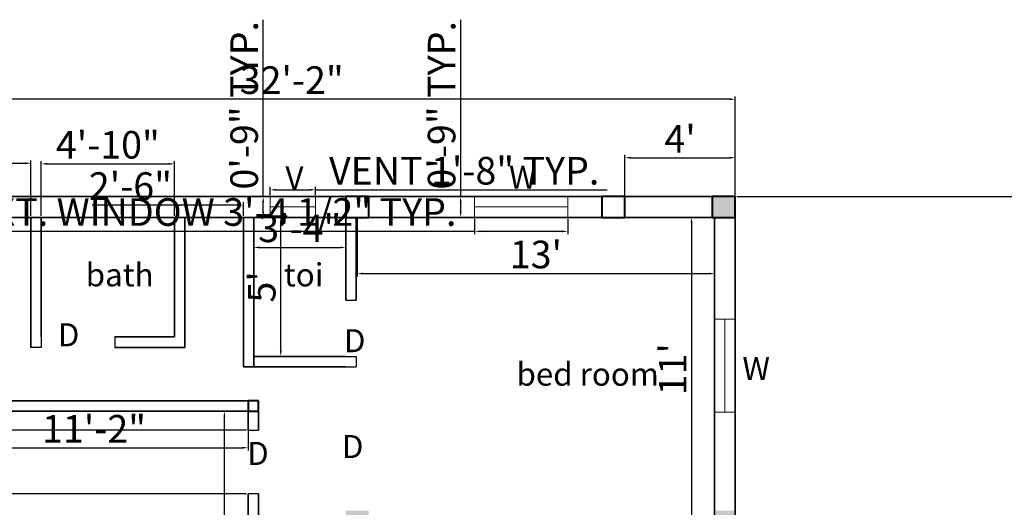
# Model space of a CAD drawing. Units: inches. Extents: x 1989 to 3287, y 1752 to 2384.
# Tile 3 of 5: x 2209 to 2638, y 2172 to 2384. Entities that reach past the tile are written whole.
import ezdxf

# ---------------------------------------------------------------- set-up
doc = ezdxf.new("R2010")
doc.units = ezdxf.units.IN
for name, color, linetype, lineweight in [('A-ANNO-DIMS', 2, 'Continuous', 18), ('A-ANNO-TEXT', 7, 'Continuous', 18), ('A-AREA-IDEN', 7, 'Continuous', 18), ('A-COLS', 1, 'Continuous', 40), ('A-COLS-PATT', 8, 'Continuous', 13), ('A-DOOR', 3, 'Continuous', 25), ('A-GLAZ', 4, 'Continuous', 18), ('A-WALL', 7, 'Continuous', 35)]:
    doc.layers.add(name, color=color, linetype=linetype, lineweight=lineweight)
doc.styles.get("Standard").update_dxf_attribs({"font": 'arial.ttf'})
doc.dimstyles.new('ISO-25', dxfattribs={"dimtxt": 12, "dimasz": 2.5, "dimexe": 1.25, "dimexo": 0.625, "dimtad": 1, "dimdec": 0, "dimlunit": 4, "dimtxsty": 'Standard', "dimcen": 2.5, "dimadec": 0, "dimazin": 0, "dimtfac": 1, "dimtdec": 0, "dimtmove": 0, "dimatfit": 3, "dimfxl": 1, "dimarcsym": 0})

# ---------------------------------------------------------------- blocks, each defined once
blk = doc.blocks.new('*D9')
at = {"layer": 'A-ANNO-DIMS', "color": 0, "lineweight": -2, "transparency": 16777216}
for p, q in [((2308.01, 2213.45), (2297.11, 2213.45)), ((2298.36, 2043.68), (2298.36, 2210.95)), ((2308.01, 2041.18), (2297.11, 2041.18))]:
    blk.add_line(p, q, dxfattribs=at)
at = {"layer": 'A-ANNO-DIMS', "color": 0, "transparency": 16777216}
for points in [[(2297.94, 2210.95), (2298.78, 2210.95), (2298.36, 2213.45)], [(2297.94, 2043.68), (2298.78, 2043.68), (2298.36, 2041.18)]]:
    blk.add_solid(points, dxfattribs=at)
at = {"layer": 'Defpoints', "color": 0, "transparency": 16777216}
for p in [(2298.36, 2213.45), (2308.64, 2213.45), (2308.64, 2041.18)]:
    blk.add_point(p, dxfattribs=at)
at = {"layer": 'A-ANNO-DIMS', "color": 0, "transparency": 16777216, "insert": (2291.71, 2127.31), "char_height": 12, "attachment_point": 5, "rotation": 90}
blk.add_mtext('14\'-4"', dxfattribs=at)
blk = doc.blocks.new('*D10')
at = {"layer": 'A-ANNO-DIMS', "color": 0, "lineweight": -2, "transparency": 16777216}
for p, q in [((2174.64, 2212.82), (2174.64, 2196.3)), ((2308.64, 2212.82), (2308.64, 2196.3)), ((2177.14, 2197.55), (2306.14, 2197.55))]:
    blk.add_line(p, q, dxfattribs=at)
at = {"layer": 'A-ANNO-DIMS', "color": 0, "transparency": 16777216}
for points in [[(2177.14, 2197.97), (2177.14, 2197.13), (2174.64, 2197.55)], [(2306.14, 2197.97), (2306.14, 2197.13), (2308.64, 2197.55)]]:
    blk.add_solid(points, dxfattribs=at)
at = {"layer": 'Defpoints', "color": 0, "transparency": 16777216}
for p in [(2174.64, 2213.45), (2308.64, 2213.45), (2308.64, 2197.55)]:
    blk.add_point(p, dxfattribs=at)
at = {"layer": 'A-ANNO-DIMS', "color": 0, "transparency": 16777216, "insert": (2241.64, 2204.2), "char_height": 12, "attachment_point": 5}
blk.add_mtext('11\'-2"', dxfattribs=at)
blk = doc.blocks.new('*D12')
at = {"layer": 'A-ANNO-DIMS', "color": 0, "lineweight": -2, "transparency": 16777216}
for p, q in [((2134.64, 2307.3), (2134.64, 2350.26)), ((2518.14, 2349.01), (2137.14, 2349.01)), ((2520.64, 2307.3), (2520.64, 2350.26))]:
    blk.add_line(p, q, dxfattribs=at)
at = {"layer": 'A-ANNO-DIMS', "color": 0, "transparency": 16777216}
for points in [[(2137.14, 2349.43), (2137.14, 2348.6), (2134.64, 2349.01)], [(2518.14, 2349.43), (2518.14, 2348.6), (2520.64, 2349.01)]]:
    blk.add_solid(points, dxfattribs=at)
at = {"layer": 'Defpoints', "color": 0, "transparency": 16777216}
for p in [(2134.64, 2349.01), (2134.64, 2306.68), (2520.64, 2306.68)]:
    blk.add_point(p, dxfattribs=at)
at = {"layer": 'A-ANNO-DIMS', "color": 0, "transparency": 16777216, "insert": (2327.64, 2355.77), "char_height": 12, "attachment_point": 5}
blk.add_mtext('32\'-2"', dxfattribs=at)
blk = doc.blocks.new('*D13')
at = {"layer": 'A-ANNO-DIMS', "color": 0, "lineweight": -2, "transparency": 16777216}
for p, q in [((2511.01, 2297.68), (2500.35, 2297.68)), ((2501.6, 2295.18), (2501.6, 2168.18)), ((2511.01, 2165.68), (2500.35, 2165.68))]:
    blk.add_line(p, q, dxfattribs=at)
at = {"layer": 'A-ANNO-DIMS', "color": 0, "transparency": 16777216}
for points in [[(2501.18, 2295.18), (2502.02, 2295.18), (2501.6, 2297.68)], [(2501.18, 2168.18), (2502.02, 2168.18), (2501.6, 2165.68)]]:
    blk.add_solid(points, dxfattribs=at)
at = {"layer": 'Defpoints', "color": 0, "transparency": 16777216}
for p in [(2511.64, 2297.68), (2501.6, 2165.68), (2511.64, 2165.68)]:
    blk.add_point(p, dxfattribs=at)
at = {"layer": 'A-ANNO-DIMS', "color": 0, "transparency": 16777216, "insert": (2494.95, 2231.68), "char_height": 12, "attachment_point": 5, "rotation": 90}
blk.add_mtext("11'", dxfattribs=at)
blk = doc.blocks.new('*D14')
at = {"layer": 'A-ANNO-DIMS', "color": 0, "lineweight": -2, "transparency": 16777216}
for p, q in [((2356.14, 2297.05), (2356.14, 2271.98)), ((2511.64, 2297.05), (2511.64, 2271.98)), ((2358.64, 2273.23), (2509.14, 2273.23))]:
    blk.add_line(p, q, dxfattribs=at)
at = {"layer": 'A-ANNO-DIMS', "color": 0, "transparency": 16777216}
for points in [[(2358.64, 2273.65), (2358.64, 2272.82), (2356.14, 2273.23)], [(2509.14, 2273.65), (2509.14, 2272.82), (2511.64, 2273.23)]]:
    blk.add_solid(points, dxfattribs=at)
at = {"layer": 'Defpoints', "color": 0, "transparency": 16777216}
for p in [(2356.14, 2297.68), (2511.64, 2297.68), (2511.64, 2273.23)]:
    blk.add_point(p, dxfattribs=at)
at = {"layer": 'A-ANNO-DIMS', "color": 0, "transparency": 16777216, "insert": (2433.89, 2279.99), "char_height": 12, "attachment_point": 5}
blk.add_mtext("13'", dxfattribs=at)
blk = doc.blocks.new('*D15')
at = {"layer": 'A-ANNO-DIMS', "color": 0, "lineweight": -2, "transparency": 16777216}
for p, q in [((2311.14, 2297.05), (2311.14, 2283.35)), ((2351.14, 2297.05), (2351.14, 2283.35)), ((2313.64, 2284.6), (2348.64, 2284.6))]:
    blk.add_line(p, q, dxfattribs=at)
at = {"layer": 'A-ANNO-DIMS', "color": 0, "transparency": 16777216}
for points in [[(2313.64, 2285.02), (2313.64, 2284.18), (2311.14, 2284.6)], [(2348.64, 2285.02), (2348.64, 2284.18), (2351.14, 2284.6)]]:
    blk.add_solid(points, dxfattribs=at)
at = {"layer": 'Defpoints', "color": 0, "transparency": 16777216}
for p in [(2311.14, 2297.68), (2351.14, 2297.68), (2351.14, 2284.6)]:
    blk.add_point(p, dxfattribs=at)
at = {"layer": 'A-ANNO-DIMS', "color": 0, "transparency": 16777216, "insert": (2331.14, 2291.36), "char_height": 12, "attachment_point": 5}
blk.add_mtext('3\'-4"', dxfattribs=at)
blk = doc.blocks.new('*D16')
at = {"layer": 'A-ANNO-DIMS', "color": 0, "lineweight": -2, "transparency": 16777216}
for p, q in [((2311.76, 2297.68), (2324.13, 2297.68)), ((2322.88, 2239.73), (2322.88, 2295.18)), ((2311.76, 2237.23), (2324.13, 2237.23))]:
    blk.add_line(p, q, dxfattribs=at)
at = {"layer": 'A-ANNO-DIMS', "color": 0, "transparency": 16777216}
for points in [[(2322.46, 2295.18), (2323.29, 2295.18), (2322.88, 2297.68)], [(2322.46, 2239.73), (2323.29, 2239.73), (2322.88, 2237.23)]]:
    blk.add_solid(points, dxfattribs=at)
at = {"layer": 'Defpoints', "color": 0, "transparency": 16777216}
for p in [(2311.14, 2297.68), (2322.88, 2297.68), (2311.14, 2237.23)]:
    blk.add_point(p, dxfattribs=at)
at = {"layer": 'A-ANNO-DIMS', "color": 0, "transparency": 16777216, "insert": (2316.15, 2267.45), "char_height": 12, "attachment_point": 5, "rotation": 90}
blk.add_mtext("5'", dxfattribs=at)
blk = doc.blocks.new('*D17')
at = {"layer": 'A-ANNO-DIMS', "color": 0, "lineweight": -2, "transparency": 16777216}
for p, q in [((2276.64, 2302.98), (2240.78, 2302.98)), ((2276.64, 2298.3), (2276.64, 2304.23)), ((2304.14, 2302.98), (2279.14, 2302.98)), ((2306.64, 2298.3), (2306.64, 2304.23))]:
    blk.add_line(p, q, dxfattribs=at)
at = {"layer": 'A-ANNO-DIMS', "color": 0, "transparency": 16777216}
for points in [[(2279.14, 2303.4), (2279.14, 2302.56), (2276.64, 2302.98)], [(2304.14, 2303.4), (2304.14, 2302.56), (2306.64, 2302.98)]]:
    blk.add_solid(points, dxfattribs=at)
at = {"layer": 'Defpoints', "color": 0, "transparency": 16777216}
for p in [(2276.64, 2302.98), (2276.64, 2297.68), (2306.64, 2297.68)]:
    blk.add_point(p, dxfattribs=at)
at = {"layer": 'A-ANNO-DIMS', "color": 0, "transparency": 16777216, "insert": (2257.46, 2309.73), "char_height": 12, "attachment_point": 5}
blk.add_mtext('2\'-6"', dxfattribs=at)
blk = doc.blocks.new('*D31')
at = {"layer": 'A-ANNO-DIMS', "color": 0, "lineweight": -2, "transparency": 16777216}
for p, q in [((2166.14, 2298.3), (2166.14, 2322.43)), ((2214.14, 2298.3), (2214.14, 2322.43)), ((2168.64, 2321.18), (2211.64, 2321.18))]:
    blk.add_line(p, q, dxfattribs=at)
at = {"layer": 'A-ANNO-DIMS', "color": 0, "transparency": 16777216}
for points in [[(2168.64, 2321.6), (2168.64, 2320.76), (2166.14, 2321.18)], [(2211.64, 2321.6), (2211.64, 2320.76), (2214.14, 2321.18)]]:
    blk.add_solid(points, dxfattribs=at)
at = {"layer": 'Defpoints', "color": 0, "transparency": 16777216}
for p in [(2214.14, 2321.18), (2166.14, 2297.68), (2214.14, 2297.68)]:
    blk.add_point(p, dxfattribs=at)
at = {"layer": 'A-ANNO-DIMS', "color": 0, "transparency": 16777216, "insert": (2190.14, 2327.8), "char_height": 12, "attachment_point": 5}
blk.add_mtext("4'", dxfattribs=at)
blk = doc.blocks.new('*D33')
at = {"layer": 'A-ANNO-DIMS', "color": 0, "lineweight": -2, "transparency": 16777216}
for p, q in [((2218.64, 2298.3), (2218.64, 2322.17)), ((2276.64, 2298.3), (2276.64, 2322.17)), ((2221.14, 2320.92), (2274.14, 2320.92))]:
    blk.add_line(p, q, dxfattribs=at)
at = {"layer": 'A-ANNO-DIMS', "color": 0, "transparency": 16777216}
for points in [[(2221.14, 2321.33), (2221.14, 2320.5), (2218.64, 2320.92)], [(2274.14, 2321.33), (2274.14, 2320.5), (2276.64, 2320.92)]]:
    blk.add_solid(points, dxfattribs=at)
at = {"layer": 'Defpoints', "color": 0, "transparency": 16777216}
for p in [(2276.64, 2320.92), (2218.64, 2297.68), (2276.64, 2297.68)]:
    blk.add_point(p, dxfattribs=at)
at = {"layer": 'A-ANNO-DIMS', "color": 0, "transparency": 16777216, "insert": (2247.64, 2327.67), "char_height": 12, "attachment_point": 5}
blk.add_mtext('4\'-10"', dxfattribs=at)
blk = doc.blocks.new('*D34')
at = {"layer": 'A-ANNO-DIMS', "color": 0, "lineweight": -2, "transparency": 16777216}
for p, q in [((2472.59, 2307.3), (2472.59, 2324.85)), ((2475.09, 2323.6), (2518.14, 2323.6)), ((2520.64, 2307.3), (2520.64, 2324.85))]:
    blk.add_line(p, q, dxfattribs=at)
at = {"layer": 'A-ANNO-DIMS', "color": 0, "transparency": 16777216}
for points in [[(2475.09, 2324.01), (2475.09, 2323.18), (2472.59, 2323.6)], [(2518.14, 2324.01), (2518.14, 2323.18), (2520.64, 2323.6)]]:
    blk.add_solid(points, dxfattribs=at)
at = {"layer": 'Defpoints', "color": 0, "transparency": 16777216}
for p in [(2520.64, 2323.6), (2472.59, 2306.68), (2520.64, 2306.68)]:
    blk.add_point(p, dxfattribs=at)
at = {"layer": 'A-ANNO-DIMS', "color": 0, "transparency": 16777216, "insert": (2496.62, 2330.22), "char_height": 12, "attachment_point": 5}
blk.add_mtext("4'", dxfattribs=at)
blk = doc.blocks.new('WIN-EXT-STANDARD')
blk.add_line((4.5, 0), (4.5, 40.55))
blk.add_lwpolyline([(0, 40.55), (9, 40.55), (9, 0), (0, 0)], close=True)
blk = doc.blocks.new('VENT-TOILET')
blk.add_line((0, 4.5), (19.78, 4.5))
blk.add_lwpolyline([(0, 0), (19.78, 0), (19.78, 9), (0, 9)], close=True)
blk = doc.blocks.new('*D53')
at = {"layer": 'A-ANNO-DIMS', "color": 0, "lineweight": -2, "transparency": 16777216}
for p, q in [((2407.24, 2297.05), (2407.24, 2290.35)), ((2447.79, 2297.05), (2447.79, 2290.35)), ((2407.24, 2291.6), (2182.88, 2291.6)), ((2445.29, 2291.6), (2409.74, 2291.6))]:
    blk.add_line(p, q, dxfattribs=at)
at = {"layer": 'A-ANNO-DIMS', "color": 0, "transparency": 16777216}
for points in [[(2409.74, 2292.01), (2409.74, 2291.18), (2407.24, 2291.6)], [(2445.29, 2292.01), (2445.29, 2291.18), (2447.79, 2291.6)]]:
    blk.add_solid(points, dxfattribs=at)
at = {"layer": 'Defpoints', "color": 0, "transparency": 16777216}
for p in [(2407.24, 2297.68), (2447.79, 2297.68), (2407.24, 2291.6)]:
    blk.add_point(p, dxfattribs=at)
at = {"layer": 'A-ANNO-DIMS', "color": 0, "transparency": 16777216, "insert": (2293.81, 2298.44), "char_height": 12, "attachment_point": 5}
blk.add_mtext('EXT. WINDOW 3\'-4 1/2" TYP.', dxfattribs=at)
blk = doc.blocks.new('*D54')
at = {"layer": 'A-ANNO-DIMS', "color": 0, "lineweight": -2, "transparency": 16777216}
for p, q in [((2401.16, 2306.68), (2401.16, 2383.58)), ((2406.62, 2306.68), (2399.91, 2306.68)), ((2401.16, 2300.18), (2401.16, 2304.18)), ((2406.62, 2297.68), (2399.91, 2297.68))]:
    blk.add_line(p, q, dxfattribs=at)
at = {"layer": 'A-ANNO-DIMS', "color": 0, "transparency": 16777216}
for points in [[(2400.74, 2304.18), (2401.58, 2304.18), (2401.16, 2306.68)], [(2400.74, 2300.18), (2401.58, 2300.18), (2401.16, 2297.68)]]:
    blk.add_solid(points, dxfattribs=at)
at = {"layer": 'Defpoints', "color": 0, "transparency": 16777216}
for p in [(2401.16, 2306.68), (2407.24, 2306.68), (2407.24, 2297.68)]:
    blk.add_point(p, dxfattribs=at)
at = {"layer": 'A-ANNO-DIMS', "color": 0, "transparency": 16777216, "insert": (2394.41, 2346.38), "char_height": 12, "attachment_point": 5, "rotation": 90}
blk.add_mtext('0\'-9" TYP.', dxfattribs=at)
blk = doc.blocks.new('*D57')
at = {"layer": 'A-ANNO-DIMS', "color": 0, "lineweight": -2, "transparency": 16777216}
for p, q in [((2318.22, 2307.3), (2318.22, 2310.9)), ((2320.72, 2309.65), (2335.5, 2309.65)), ((2338, 2307.3), (2338, 2310.9)), ((2338, 2309.65), (2464.88, 2309.65))]:
    blk.add_line(p, q, dxfattribs=at)
at = {"layer": 'A-ANNO-DIMS', "color": 0, "transparency": 16777216}
for points in [[(2320.72, 2310.06), (2320.72, 2309.23), (2318.22, 2309.65)], [(2335.5, 2310.06), (2335.5, 2309.23), (2338, 2309.65)]]:
    blk.add_solid(points, dxfattribs=at)
at = {"layer": 'Defpoints', "color": 0, "transparency": 16777216}
for p in [(2338, 2309.65), (2318.22, 2306.68), (2338, 2306.68)]:
    blk.add_point(p, dxfattribs=at)
at = {"layer": 'A-ANNO-DIMS', "color": 0, "transparency": 16777216, "insert": (2402.69, 2316.4), "char_height": 12, "attachment_point": 5}
blk.add_mtext('VENT 1\'-8" TYP.', dxfattribs=at)
blk = doc.blocks.new('*D58')
at = {"layer": 'A-ANNO-DIMS', "color": 0, "lineweight": -2, "transparency": 16777216}
for p, q in [((2315.25, 2306.68), (2315.25, 2383.58)), ((2317.59, 2306.68), (2314, 2306.68)), ((2315.25, 2300.18), (2315.25, 2304.18)), ((2317.59, 2297.68), (2314, 2297.68))]:
    blk.add_line(p, q, dxfattribs=at)
at = {"layer": 'A-ANNO-DIMS', "color": 0, "transparency": 16777216}
for points in [[(2314.83, 2304.18), (2315.67, 2304.18), (2315.25, 2306.68)], [(2314.83, 2300.18), (2315.67, 2300.18), (2315.25, 2297.68)]]:
    blk.add_solid(points, dxfattribs=at)
at = {"layer": 'Defpoints', "color": 0, "transparency": 16777216}
for p in [(2315.25, 2306.68), (2318.22, 2306.68), (2318.22, 2297.68)]:
    blk.add_point(p, dxfattribs=at)
at = {"layer": 'A-ANNO-DIMS', "color": 0, "transparency": 16777216, "insert": (2308.5, 2346.38), "char_height": 12, "attachment_point": 5, "rotation": 90}
blk.add_mtext('0\'-9" TYP.', dxfattribs=at)
blk = doc.blocks.new('*D64')
at = {"layer": 'A-ANNO-DIMS', "color": 0, "lineweight": -2, "transparency": 16777216}
for p, q in [((2521.26, 2306.68), (3180.41, 2306.68)), ((3179.16, 1876.18), (3179.16, 2304.18)), ((2379.26, 1873.68), (3180.41, 1873.68))]:
    blk.add_line(p, q, dxfattribs=at)
at = {"layer": 'A-ANNO-DIMS', "color": 0, "transparency": 16777216}
for points in [[(3178.74, 2304.18), (3179.58, 2304.18), (3179.16, 2306.68)], [(3178.74, 1876.18), (3179.58, 1876.18), (3179.16, 1873.68)]]:
    blk.add_solid(points, dxfattribs=at)
at = {"layer": 'Defpoints', "color": 0, "transparency": 16777216}
for p in [(2520.64, 2306.68), (3179.16, 2306.68), (2378.64, 1873.68)]:
    blk.add_point(p, dxfattribs=at)
at = {"layer": 'A-ANNO-DIMS', "color": 0, "transparency": 16777216, "insert": (3172.4, 2090.18), "char_height": 12, "attachment_point": 5, "rotation": 90}
blk.add_mtext('36\'-1"', dxfattribs=at)
blk = doc.blocks.new('*D75')
at = {"layer": 'A-ANNO-DIMS', "color": 0, "lineweight": -2, "transparency": 16777216}
for p, q in [((2013.54, 2205.2), (2013.54, 2269.02)), ((2308.01, 2205.2), (2012.29, 2205.2)), ((2013.54, 2179.95), (2013.54, 2202.7)), ((2308.01, 2177.45), (2012.29, 2177.45))]:
    blk.add_line(p, q, dxfattribs=at)
at = {"layer": 'A-ANNO-DIMS', "color": 0, "transparency": 16777216}
for points in [[(2013.12, 2202.7), (2013.95, 2202.7), (2013.54, 2205.2)], [(2013.12, 2179.95), (2013.95, 2179.95), (2013.54, 2177.45)]]:
    blk.add_solid(points, dxfattribs=at)
at = {"layer": 'Defpoints', "color": 0, "transparency": 16777216}
for p in [(2013.54, 2205.2), (2308.64, 2205.2), (2308.64, 2177.45)]:
    blk.add_point(p, dxfattribs=at)
at = {"layer": 'A-ANNO-DIMS', "color": 0, "transparency": 16777216, "insert": (2006.7, 2238.36), "char_height": 12, "attachment_point": 5, "rotation": 90}
blk.add_mtext('2\'-3 1/2"', dxfattribs=at)

msp = doc.modelspace()

# ---------------------------------------------------------------- hatches: boundary and pattern name
at = {"layer": 'A-COLS-PATT'}
h = msp.add_hatch(dxfattribs=at)
h.set_pattern_fill('GRAVEL', color=256, scale=0.2)
h.paths.add_polyline_path([(3123.21, 2045.68), (3114.21, 2045.68), (3114.21, 2041.18), (3113.21, 2041.18), (3113.21, 2036.68), (3123.21, 2036.68)])
h.paths.add_polyline_path([(2962.75, 2170.18), (2952.75, 2170.18), (2952.75, 2161.18), (2962.75, 2161.18)])
h.paths.add_polyline_path([(2520.59, 2306.68), (2510.59, 2306.68), (2510.59, 2297.68), (2520.59, 2297.68)])
h.paths.add_polyline_path([(2520.64, 2170.18), (2511.64, 2170.18), (2511.64, 2161.18), (2520.64, 2161.18)])
h.paths.add_polyline_path([(2364.99, 2045.68), (2354.99, 2045.68), (2354.99, 2036.68), (2364.99, 2036.68)])
h.paths.add_polyline_path([(2361.14, 2170.18), (2351.14, 2170.18), (2351.14, 2161.18), (2361.14, 2161.18)])
h = msp.add_hatch(dxfattribs=at)
h.set_pattern_fill('GRAVEL', color=256, scale=0.2)
h.paths.add_polyline_path([(2520.64, 2045.68), (2511.64, 2045.68), (2511.64, 2041.18), (2510.64, 2041.18), (2510.64, 2036.68), (2520.64, 2036.68)])
h.paths.add_polyline_path([(2520.63, 1966.68), (2510.63, 1966.68), (2510.63, 1957.68), (2520.63, 1957.68)])
h.paths.add_polyline_path([(2323.14, 1882.68), (2313.14, 1882.68), (2313.14, 1873.68), (2323.14, 1873.68)])
h.paths.add_polyline_path([(2378.64, 1882.68), (2368.64, 1882.68), (2368.64, 1873.68), (2378.64, 1873.68)])
h.paths.add_polyline_path([(2378.64, 1966.68), (2368.64, 1966.68), (2368.64, 1957.68), (2378.64, 1957.68)])
h.paths.add_polyline_path([(2323.14, 1966.68), (2313.14, 1966.68), (2313.14, 1957.68), (2323.14, 1957.68)])
h.paths.add_polyline_path([(2313.14, 2041.18), (2308.64, 2041.18), (2308.64, 2036.68), (2313.14, 2036.68)])
h.paths.add_polyline_path([(2304.29, 2102.44), (2304.29, 2151.15), (2279.56, 2151.15), (2279.56, 2102.44)], flags=9)
h.paths.add_polyline_path([(2216.76, 2191.62), (2265.47, 2191.62), (2265.47, 2216.35), (2216.76, 2216.35)], flags=9)
h.paths.add_polyline_path([(2507.53, 2217.24), (2507.53, 2245.08), (2482.8, 2245.08), (2482.8, 2217.24)], flags=9)
h.paths.add_polyline_path([(2466.45, 2144.02), (2484.98, 2144.02), (2484.98, 2168.75), (2466.45, 2168.75)], flags=9)
h.paths.add_polyline_path([(2462.3, 2086.74), (2462.3, 2114.58), (2437.57, 2114.58), (2437.57, 2086.74)], flags=9)
h.paths.add_polyline_path([(2349.26, 2050.52), (2397.97, 2050.52), (2397.97, 2075.25), (2349.26, 2075.25)], flags=9)
h.paths.add_polyline_path([(2432.27, 2086.74), (2432.27, 2114.58), (2407.54, 2114.58), (2407.54, 2086.74)], flags=9)
h.paths.add_polyline_path([(2304.67, 2184.6), (2319.75, 2184.6), (2319.75, 2205.2), (2304.67, 2205.2)], flags=9)
h.paths.add_polyline_path([(2345.88, 2187.62), (2360.97, 2187.62), (2360.97, 2208.22), (2345.88, 2208.22)], flags=9)
h.paths.add_polyline_path([(2429.95, 2091.23), (2445.03, 2091.23), (2445.03, 2111.84), (2429.95, 2111.84)], flags=9)
h.paths.add_polyline_path([(2346.78, 2233.62), (2361.86, 2233.62), (2361.86, 2254.22), (2346.78, 2254.22)], flags=9)
h.paths.add_polyline_path([(2222.31, 2236.18), (2237.39, 2236.18), (2237.39, 2256.78), (2222.31, 2256.78)], flags=9)
h.paths.add_polyline_path([(2186.25, 2233.03), (2201.34, 2233.03), (2201.34, 2253.64), (2186.25, 2253.64)], flags=9)
h.paths.add_polyline_path([(2356.5, 2089.75), (2417.39, 2089.75), (2417.39, 2110.36), (2356.5, 2110.36)], flags=9)
h.paths.add_polyline_path([(2450.78, 2087.89), (2500.04, 2087.89), (2500.04, 2108.49), (2450.78, 2108.49)], flags=9)
h.paths.add_polyline_path([(2226.77, 2120.65), (2286.89, 2120.65), (2286.89, 2141.25), (2226.77, 2141.25)], flags=9)
h.paths.add_polyline_path([(2422.03, 2219.06), (2486.03, 2219.06), (2486.03, 2239.67), (2422.03, 2239.67)], flags=9)
h.paths.add_polyline_path([(2321.5, 2262.24), (2341.25, 2262.24), (2341.25, 2282.84), (2321.5, 2282.84)], flags=9)
h.paths.add_polyline_path([(2234.58, 2262.24), (2266.77, 2262.24), (2266.77, 2282.84), (2234.58, 2282.84)], flags=9)
h.paths.add_polyline_path([(2179.85, 2262.24), (2199.6, 2262.24), (2199.6, 2282.84), (2179.85, 2282.84)], flags=9)

# ---------------------------------------------------------------- linework, layer by layer
at = {"layer": 'A-COLS'}
for points in [[(2351.14, 2297.68), (2361.14, 2297.68), (2361.14, 2306.68), (2351.14, 2306.68)], [(2462.59, 2297.68), (2472.59, 2297.68), (2472.59, 2306.68), (2462.59, 2306.68)], [(2510.59, 2297.68), (2520.59, 2297.68), (2520.59, 2306.68), (2510.59, 2306.68)], [(2313.14, 2217.95), (2308.64, 2217.95), (2308.64, 2213.45), (2313.14, 2213.45)]]:
    msp.add_lwpolyline(points, close=True, dxfattribs=at)
at = {"layer": 'A-DOOR'}
for p, q in [((2351.14, 2261.68), (2355.64, 2261.68)), ((2214.14, 2241.18), (2214.14, 2245.68)), ((2218.64, 2245.68), (2218.64, 2241.18)), ((2250.64, 2245.68), (2250.64, 2241.18)), ((2218.64, 2241.18), (2214.14, 2241.18)), ((2351.14, 2237.23), (2355.64, 2237.23)), ((2355.64, 2237.23), (2355.64, 2232.73)), ((2351.14, 2232.73), (2355.64, 2232.73))]:
    msp.add_line(p, q, dxfattribs=at)
for points in [[(2308.64, 2205.2), (2313.14, 2205.2)], [(2313.14, 2177.45), (2308.64, 2177.45)]]:
    msp.add_lwpolyline(points, dxfattribs=at)
at = {"layer": 'A-WALL'}
for p, q in [((2214.14, 2297.68), (2166.14, 2297.68)), ((2214.14, 2241.18), (2214.14, 2297.68)), ((2218.64, 2245.68), (2218.64, 2297.68)), ((2218.64, 2297.68), (2218.64, 2273.65)), ((2306.64, 2297.68), (2276.64, 2297.68)), ((2276.64, 2297.68), (2276.64, 2245.68)), ((2281.14, 2297.68), (2281.14, 2241.18)), ((2306.64, 2297.68), (2306.64, 2232.73)), ((2351.14, 2297.68), (2311.14, 2297.68)), ((2311.14, 2297.68), (2311.14, 2232.73)), ((2351.14, 2297.68), (2351.14, 2261.68)), ((2511.64, 2297.68), (2355.64, 2297.68)), ((2355.64, 2297.68), (2355.64, 2261.68)), ((2276.64, 2245.68), (2250.64, 2245.68)), ((2281.14, 2241.18), (2250.64, 2241.18)), ((2311.14, 2237.23), (2351.14, 2237.23)), ((2306.64, 2232.73), (2351.14, 2232.73)), ((2313.14, 2217.95), (2165.64, 2217.95)), ((2313.14, 2217.95), (2313.14, 2205.2)), ((2308.64, 2213.45), (2174.64, 2213.45)), ((2308.64, 2213.45), (2308.64, 2205.2)), ((2308.64, 2177.45), (2308.64, 2099.68)), ((2313.14, 2177.45), (2313.14, 2099.68))]:
    msp.add_line(p, q, dxfattribs=at)
for points in [[(2520.64, 2090.68), (2520.64, 2306.68), (2134.64, 2306.68), (2134.64, 2137.49)], [(2511.64, 2099.68), (2511.64, 2297.68), (2143.64, 2297.68)]]:
    msp.add_lwpolyline(points, dxfattribs=at)

# ---------------------------------------------------------------- block references
at = {"layer": 'A-GLAZ'}
for name, p in [('VENT-TOILET', (2318.22, 2297.68)), ('WIN-EXT-STANDARD', (2511.64, 2212.94))]:
    msp.add_blockref(name, p, dxfattribs=at)
at = {"layer": 'A-GLAZ', "rotation": 90.00000000000011}
msp.add_blockref('WIN-EXT-STANDARD', (2447.79, 2297.68), dxfattribs=at)

# ---------------------------------------------------------------- texts
at = {"layer": 'A-ANNO-TEXT', "char_height": 10, "attachment_point": 1}
for s, insert in [('V', (2324.91, 2319.8)), ('W', (2422.18, 2320.16)), ('D', (2225.88, 2251.63)), ('D', (2350.35, 2249.07)), ('W', (2523.74, 2236.97)), ('D', (2349.46, 2203.07)), ('D', (2308.25, 2200.06))]:
    msp.add_mtext_dynamic_manual_height_columns(s, width=78.3523, gutter_width=49.99, heights=[0], dxfattribs=dict(at, insert=insert))
at = {"layer": 'A-AREA-IDEN', "char_height": 9.998, "attachment_point": 1}
for s, insert in [('bath', (2238, 2277.69)), ('toi', (2324.25, 2277.69)), ('bed room', (2425.44, 2234.52))]:
    msp.add_mtext_dynamic_manual_height_columns(s, width=78.3523, gutter_width=49.99, heights=[0], dxfattribs=dict(at, insert=insert))

# ---------------------------------------------------------------- dimensions: what is measured, and where the dimension line sits
at = {"layer": 'A-ANNO-DIMS'}
for base, p1, p2, angle, text, picture, middle in [((2315.25, 2306.68), (2318.22, 2297.68), (2318.22, 2306.68), 90, '<> TYP.', '*D58', (2308.5, 2346.38)), ((2401.16, 2306.68), (2407.24, 2297.68), (2407.24, 2306.68), 90, '<> TYP.', '*D54', (2394.41, 2346.38)), ((2407.2411, 2291.5978), (2447.789, 2297.68), (2407.2411, 2297.68), 180, 'EXT. WINDOW <> TYP.', '*D53', (2293.8119, 2298.4356))]:
    dim = msp.add_linear_dim(base=base, p1=p1, p2=p2, angle=angle, text=text, dimstyle='ISO-25', override={"dimdec": 1, "dimlfac": 1, "dimrnd": 0, "dimzin": 1, "dimdsep": 46, "dimlunit": 4, "dimfrac": 2}, dxfattribs=at)
    dim.commit()
    dim.dimension.update_dxf_attribs({"geometry": picture, "text_midpoint": middle})
for base, p1, p2, picture, middle in [((2134.64, 2349.01), (2520.64, 2306.68), (2134.64, 2306.68), '*D12', (2327.64, 2355.77)), ((2214.14, 2321.18), (2166.14, 2297.68), (2214.14, 2297.68), '*D31', (2190.14, 2327.8)), ((2276.64, 2320.92), (2218.64, 2297.68), (2276.64, 2297.68), '*D33', (2247.64, 2327.67)), ((2520.64, 2323.6), (2472.59, 2306.68), (2520.64, 2306.68), '*D34', (2496.62, 2330.22)), ((2276.64, 2302.98), (2306.64, 2297.68), (2276.64, 2297.68), '*D17', (2257.46, 2309.73)), ((2351.14, 2284.6), (2311.14, 2297.68), (2351.14, 2297.68), '*D15', (2331.14, 2291.36)), ((2511.63646977, 2273.23166677), (2356.13646977, 2297.67998165), (2511.63646977, 2297.67998165), '*D14', (2433.88646977, 2279.98763539)), ((2308.64, 2197.55), (2174.64, 2213.45), (2308.64, 2213.45), '*D10', (2241.64, 2204.2))]:
    dim = msp.add_linear_dim(base=base, p1=p1, p2=p2, dimstyle='ISO-25', override={"dimclrd": 0, "dimclre": 0, "dimclrt": 0}, dxfattribs=at)
    dim.commit()
    dim.dimension.update_dxf_attribs({"geometry": picture, "text_midpoint": middle})
dim = msp.add_linear_dim(base=(2338, 2309.65), p1=(2318.22, 2306.68), p2=(2338, 2306.68), text='VENT <> TYP.', dimstyle='ISO-25', override={"dimdec": 1, "dimlfac": 1, "dimrnd": 0, "dimzin": 1, "dimdsep": 46, "dimlunit": 4, "dimfrac": 2}, dxfattribs=at)
dim.commit()
dim.dimension.update_dxf_attribs({"geometry": '*D57', "text_midpoint": (2402.69, 2316.4)})
for base, p1, p2, override, picture, middle in [((3179.16, 2306.68), (2378.64, 1873.68), (2520.64, 2306.68), {"dimdec": 1, "dimlfac": 1, "dimrnd": 0, "dimzin": 1, "dimdsep": 46, "dimlunit": 4, "dimfrac": 2}, '*D64', (3172.4, 2090.18)), ((2322.88, 2297.68), (2311.14, 2237.23), (2311.14, 2297.68), {"dimclrd": 0, "dimclre": 0, "dimclrt": 0}, '*D16', (2316.15, 2267.45)), ((2501.6, 2165.68), (2511.64, 2297.68), (2511.64, 2165.68), {"dimclrd": 0, "dimclre": 0, "dimclrt": 0}, '*D13', (2494.95, 2231.68)), ((2013.5352, 2205.2028), (2308.6365, 2177.4539), (2308.6365, 2205.2028), {"dimdec": 1, "dimlfac": 1, "dimrnd": 0, "dimzin": 1, "dimdsep": 46, "dimlunit": 4, "dimfrac": 2}, '*D75', (2006.7015, 2238.3605)), ((2298.36, 2213.45), (2308.64, 2041.18), (2308.64, 2213.45), {"dimclrd": 0, "dimclre": 0, "dimclrt": 0}, '*D9', (2291.71, 2127.31))]:
    dim = msp.add_linear_dim(base=base, p1=p1, p2=p2, angle=90, dimstyle='ISO-25', override=override, dxfattribs=at)
    dim.commit()
    dim.dimension.update_dxf_attribs({"geometry": picture, "text_midpoint": middle})

doc.saveas('drawing.dxf')
